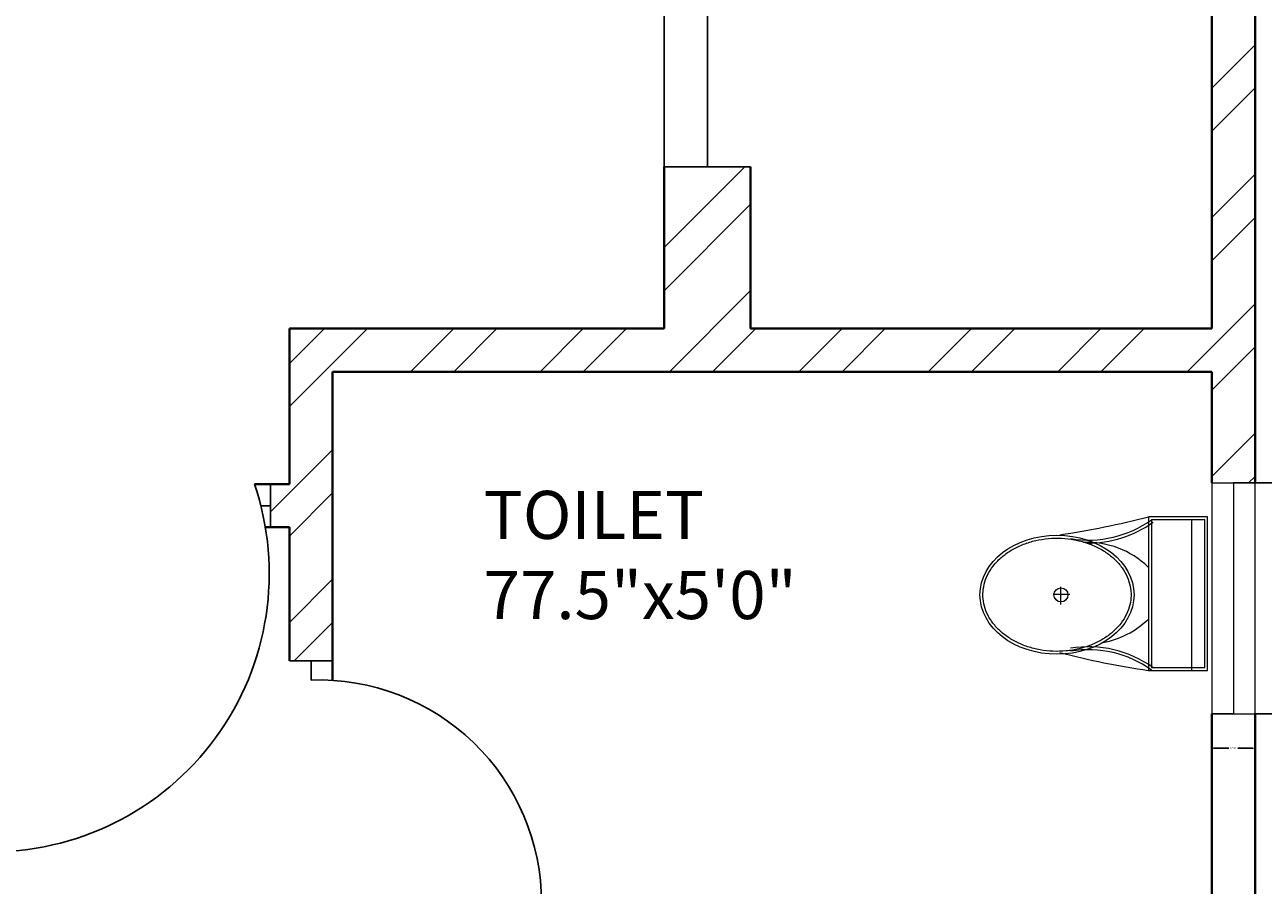
# Model space of a CAD drawing. Units: inches. Extents: x 1601 to 2297, y 1496 to 2631.
# Tile 49 of 57: x 2102 to 2231, y 2237 to 2327. Entities that reach past the tile are written whole.
import ezdxf

# ---------------------------------------------------------------- set-up
doc = ezdxf.new("R2010")
doc.units = ezdxf.units.IN
for name, color, linetype, lineweight in [('A-ANNO-DIMS', 2, 'Continuous', 18), ('A-AREA-IDEN', 7, 'Continuous', 18), ('A-DOOR', 21, 'Continuous', 25), ('A-FLOR-FIXT', 9, 'Continuous', 20), ('A-GLAZ', 161, 'Continuous', 20), ('A-WALL', 7, 'Continuous', 40), ('A-WALL-PATT', 215, 'Continuous', 13)]:
    doc.layers.add(name, color=color, linetype=linetype, lineweight=lineweight)
doc.styles.get("Standard").update_dxf_attribs({"font": 'arial.ttf'})
doc.dimstyles.get("Standard").update_dxf_attribs({"dimtxt": 0.18, "dimasz": 0.18, "dimexe": 0.18, "dimexo": 0.0625, "dimgap": 0.09, "dimtad": 0, "dimtih": 1, "dimtoh": 1, "dimdec": 4, "dimzin": 0, "dimdsep": 46, "dimtxsty": 'Standard', "dimcen": 0.09, "dimadec": 0, "dimazin": 0, "dimtfac": 1, "dimtdec": 4, "dimtofl": 0, "dimtmove": 0, "dimatfit": 3, "dimfxl": 1, "dimtolj": 1, "dimtzin": 0, "dimarcsym": 0})

# ---------------------------------------------------------------- blocks, each defined once
blk = doc.blocks.new('A$C31115884')
for p, q in [((257.5, 466.4), (257.5, 523.2)), ((283.1, 497.7), (223.4, 497.7)), ((0, 200), (0, 0)), ((520, 200), (0, 200)), ((10, 190), (10, 10)), ((510, 190), (10, 190)), ((510, 10), (510, 190)), ((520, 0), (520, 200)), ((510, 54.5), (0, 54.5)), ((10, 10), (510, 10)), ((0, 0), (520, 0))]:
    blk.add_line(p, q)
blk.add_circle((255.6, 496.4), 23.6)
for centre, radius, start, end in [((2777.7, -204.6), 2807, 165.4549, 171.7133), ((-294.5, 403.3), 364.7, 324.2091, 9.3499), ((-294.5, 403.3), 374.7, 324.2091, 9.3499), ((805.8, 403.3), 364.7, 170.6501, 215.7909), ((3237, 905), 2807, 188.2867, 194.5451), ((139.5, 406.2), 293.5, 315.8436, 2.6563), ((805.8, 403.3), 374.7, 179.2036, 215.7909), ((383.6, 406.2), 293.5, 190.2774, 224.1564)]:
    blk.add_arc(centre, radius, start, end)
blk.add_ellipse((256.2, 509.9), major_axis=(0, -260.7), ratio=0.772727)
blk.add_open_spline([(256.2, 259.2), (263.1, 259.2), (270, 259.7), (287.8, 262.3), (298.7, 265.1), (319.9, 273.1), (330.2, 278.4), (350.1, 291.1), (359.7, 298.7), (377.7, 315.9), (386.2, 325.5), (401.7, 346.6), (408.8, 358.1), (421.3, 382.5), (426.8, 395.5), (435.9, 422.4), (439.5, 436.4), (444.8, 465.1), (446.5, 479.7), (447.9, 509.2), (447.6, 524), (445, 553.3), (442.7, 567.8), (436.3, 596), (432.1, 609.7), (421.9, 636), (416, 648.6), (402.5, 672.1), (395, 683), (378.6, 703), (369.8, 712.1), (351.1, 728), (341.3, 734.8), (320.9, 746.2), (310.4, 750.7), (288.9, 757.3), (278, 759.4), (256, 761), (245, 760.6), (223.1, 757.2), (212.3, 754.3), (191.1, 746.1), (180.8, 740.7), (160.9, 727.8), (151.4, 720.1), (133.5, 702.7), (125.1, 693), (109.6, 671.7), (102.6, 660.2), (90.2, 635.7), (84.9, 622.7), (76, 595.6), (72.4, 581.6), (67.2, 552.9), (65.6, 538.2), (64.4, 508.8), (64.8, 494), (67.5, 464.7), (69.9, 450.2), (76.6, 422), (80.8, 408.3), (91.1, 382.2), (97.2, 369.7), (110.8, 346.3), (118.4, 335.4), (134.8, 315.6), (143.7, 306.7), (162.4, 290.9), (172.3, 284.2), (192.8, 273), (203.3, 268.6), (224.8, 262.2), (235.8, 260.2), (249.9, 259.3), (253, 259.2), (256.2, 259.2)], degree=3, knots=[0, 0, 0, 0, 0.110105, 0.110105, 0.285049, 0.285049, 0.459994, 0.459994, 0.634938, 0.634938, 0.809882, 0.809882, 0.984827, 0.984827, 1.159771, 1.159771, 1.334715, 1.334715, 1.50966, 1.50966, 1.684604, 1.684604, 1.859549, 1.859549, 2.034493, 2.034493, 2.209437, 2.209437, 2.384382, 2.384382, 2.559326, 2.559326, 2.73427, 2.73427, 2.909215, 2.909215, 3.084159, 3.084159, 3.259103, 3.259103, 3.434048, 3.434048, 3.608992, 3.608992, 3.783936, 3.783936, 3.958881, 3.958881, 4.133825, 4.133825, 4.30877, 4.30877, 4.483714, 4.483714, 4.658658, 4.658658, 4.833603, 4.833603, 5.008547, 5.008547, 5.183491, 5.183491, 5.358436, 5.358436, 5.53338, 5.53338, 5.708324, 5.708324, 5.883269, 5.883269, 6.058213, 6.058213, 6.233158, 6.233158, 6.283185, 6.283185, 6.283185, 6.283185])
blk = doc.blocks.new('WIN-24IN-JAMB4P5')
for p, q in [((0, 24), (4.5, 24)), ((0, 24), (0, 0)), ((4.5, 24), (2.25, 24)), ((2.25, 24), (2.25, 0)), ((4.5, 24), (4.5, 0)), ((2.25, 0), (0, 0)), ((0, 0), (4.5, 0))]:
    blk.add_line(p, q)
blk = doc.blocks.new('*D22')
at = {"layer": 'A-ANNO-DIMS', "color": 0, "lineweight": -2, "transparency": 16777216}
for p, q in [((2230.6, 2279.25), (2234.32, 2279.25)), ((2234.14, 2279.07), (2234.14, 2267.43)), ((2234.14, 2255.43), (2234.14, 2267.06)), ((2230.6, 2255.25), (2234.32, 2255.25))]:
    blk.add_line(p, q, dxfattribs=at)
at = {"layer": 'A-ANNO-DIMS', "color": 0, "transparency": 16777216}
for points in [[(2234.11, 2279.07), (2234.17, 2279.07), (2234.14, 2279.25)], [(2234.11, 2255.43), (2234.17, 2255.43), (2234.14, 2255.25)]]:
    blk.add_solid(points, dxfattribs=at)
at = {"layer": 'Defpoints', "color": 0, "transparency": 16777216}
for p in [(2230.54, 2279.25), (2234.14, 2279.25), (2230.54, 2255.25)]:
    blk.add_point(p, dxfattribs=at)
at = {"layer": 'A-ANNO-DIMS', "color": 0, "transparency": 16777216, "insert": (2234.14, 2267.25), "char_height": 0.18, "attachment_point": 5}
blk.add_mtext('\\A1;WINDOW 24 TYP.', dxfattribs=at)
blk = doc.blocks.new('*D23')
at = {"layer": 'A-ANNO-DIMS', "color": 0, "lineweight": -2, "transparency": 16777216}
for p, q in [((2226.04, 2255.18), (2226.04, 2251.47)), ((2230.54, 2255.18), (2230.54, 2251.47)), ((2226.22, 2251.65), (2227.83, 2251.65)), ((2230.36, 2251.65), (2228.75, 2251.65))]:
    blk.add_line(p, q, dxfattribs=at)
at = {"layer": 'A-ANNO-DIMS', "color": 0, "transparency": 16777216}
for points in [[(2226.22, 2251.68), (2226.22, 2251.62), (2226.04, 2251.65)], [(2230.36, 2251.68), (2230.36, 2251.62), (2230.54, 2251.65)]]:
    blk.add_solid(points, dxfattribs=at)
at = {"layer": 'Defpoints', "color": 0, "transparency": 16777216}
for p in [(2226.04, 2255.25), (2230.54, 2255.25), (2230.54, 2251.65)]:
    blk.add_point(p, dxfattribs=at)
at = {"layer": 'A-ANNO-DIMS', "color": 0, "transparency": 16777216, "insert": (2228.29, 2251.65), "char_height": 0.18, "attachment_point": 5}
blk.add_mtext('\\A1;5 TYP.', dxfattribs=at)
blk = doc.blocks.new('*D29')
at = {"layer": 'A-ANNO-DIMS', "color": 0, "lineweight": -2, "transparency": 16777216}
for p, q in [((2230.6, 2532.33), (2279.27, 2532.33)), ((2279.09, 2532.15), (2279.09, 2084.01)), ((2279.09, 1635.51), (2279.09, 2083.64)), ((2230.6, 1635.33), (2279.27, 1635.33))]:
    blk.add_line(p, q, dxfattribs=at)
at = {"layer": 'A-ANNO-DIMS', "color": 0, "transparency": 16777216}
for points in [[(2279.06, 2532.15), (2279.12, 2532.15), (2279.09, 2532.33)], [(2279.06, 1635.51), (2279.12, 1635.51), (2279.09, 1635.33)]]:
    blk.add_solid(points, dxfattribs=at)
at = {"layer": 'Defpoints', "color": 0, "transparency": 16777216}
for p in [(2230.54, 2532.33), (2279.09, 2532.33), (2230.54, 1635.33)]:
    blk.add_point(p, dxfattribs=at)
at = {"layer": 'A-ANNO-DIMS', "color": 0, "transparency": 16777216, "insert": (2279.09, 2083.83), "char_height": 0.18, "attachment_point": 5}
blk.add_mtext('\\A1;897', dxfattribs=at)

msp = doc.modelspace()

# ---------------------------------------------------------------- hatches: boundary and pattern name
at = {"layer": 'A-WALL-PATT'}
h = msp.add_hatch(dxfattribs=at)
h.set_pattern_fill('ANSI32', color=256)
h.paths.add_polyline_path([(1842.0336, 2528.0767), (1842.0336, 2532.3254), (1686.0373, 2532.3254), (1686.0373, 2492.9493), (1695.0373, 2492.9493), (1695.0373, 2523.3254), (1827.0373, 2523.3254), (1827.0373, 2416.8254), (1834.6225, 2416.8254), (1834.6225, 2419.0754), (1834.6225, 2421.3254), (1831.5373, 2421.3254), (1831.5373, 2523.3254), (1842.0336, 2523.3254)])
h.paths.add_polyline_path([(1695.0373, 2432.9493), (1686.0373, 2432.9493), (1686.0373, 2325.989), (1695.0373, 2325.989), (1695.0373, 2347.8254), (1827.0373, 2347.8254), (1827.0373, 2287.8254), (1823.2991, 2287.8254), (1823.2991, 2283.3254), (1847.9422, 2283.3254), (1847.9422, 2285.5754), (1847.9422, 2287.8254), (1831.5373, 2287.8254), (1831.5373, 2347.8254), (1846.9946, 2347.8254), (1846.9946, 2350.0754), (1846.9946, 2352.3254), (1695.0373, 2352.3254)])
h.paths.add_polyline_path([(1807.1169, 1573.5395), (2055.0405, 1573.5395), (2055.0405, 1610.6322), (1807.1169, 1610.6322)], flags=9)
h.paths.add_polyline_path([(1841.1631, 1712.7967), (1870.3957, 1712.7967), (1870.3957, 1731.454), (1841.1631, 1731.454)], flags=9)
h.paths.add_polyline_path([(2144.3862, 1772.185), (2191.0233, 1772.185), (2191.0233, 1790.8423), (2144.3862, 1790.8423)], flags=9)
h.paths.add_polyline_path([(2143.0128, 1827.3312), (2177.9958, 1827.3312), (2177.9958, 1845.9886), (2143.0128, 1845.9886)], flags=9)
h.paths.add_polyline_path([(2041.2439, 1833.5691), (2070.8516, 1833.5691), (2070.8516, 1852.2264), (2041.2439, 1852.2264)], flags=9)
h.paths.add_polyline_path([(2097.2791, 1947.0598), (2134.2061, 1947.0598), (2134.2061, 1965.7171), (2097.2791, 1965.7171)], flags=9)
h.paths.add_polyline_path([(2214.995, 1904.3124), (2214.995, 1942.2899), (2196.3376, 1942.2899), (2196.3376, 1904.3124)], flags=9)
h.paths.add_polyline_path([(2186.6284, 2043.8031), (2219.7935, 2043.8031), (2219.7935, 2062.4605), (2186.6284, 2062.4605)], flags=9)
h.paths.add_polyline_path([(2064.0877, 2031.616), (2097.4949, 2031.616), (2097.4949, 2050.2734), (2064.0877, 2050.2734)], flags=9)
h.paths.add_polyline_path([(1973.1349, 1986.0688), (2008.4009, 1986.0688), (2008.4009, 2004.7261), (1973.1349, 2004.7261)], flags=9)
h.paths.add_polyline_path([(1976.3676, 2106.9635), (2005.7469, 2106.9635), (2005.7469, 2125.6209), (1976.3676, 2125.6209)], flags=9)
h.paths.add_polyline_path([(1991.7852, 2180.4863), (2027.0513, 2180.4863), (2027.0513, 2199.1437), (1991.7852, 2199.1437)], flags=9)
h.paths.add_polyline_path([(2106.1801, 2187.9359), (2152.2101, 2187.9359), (2152.2101, 2206.5932), (2106.1801, 2206.5932)], flags=9)
h.paths.add_polyline_path([(2148.6686, 2262.2542), (2182.318, 2262.2542), (2182.318, 2280.9115), (2148.6686, 2280.9115)], flags=9)
h.paths.add_polyline_path([(2041.6327, 2252.8147), (2071.2405, 2252.8147), (2071.2405, 2271.4721), (2041.6327, 2271.4721)], flags=9)
h.paths.add_polyline_path([(2063.9734, 2375.4265), (2100.9004, 2375.4265), (2100.9004, 2394.0839), (2063.9734, 2394.0839)], flags=9)
h.paths.add_polyline_path([(2216.4955, 2330.9748), (2216.4955, 2370.2654), (2197.8381, 2370.2654), (2197.8381, 2330.9748)], flags=9)
h.paths.add_polyline_path([(2179.1416, 2485.8687), (2212.3067, 2485.8687), (2212.3067, 2504.5261), (2179.1416, 2504.5261)], flags=9)
h.paths.add_polyline_path([(2078.7442, 2471.1516), (2112.1514, 2471.1516), (2112.1514, 2489.809), (2078.7442, 2489.809)], flags=9)
h.paths.add_polyline_path([(1915.9631, 2329.4668), (1952.8902, 2329.4668), (1952.8902, 2348.1241), (1915.9631, 2348.1241)], flags=9)
h.paths.add_polyline_path([(1904.3189, 2499.6709), (1940.4512, 2499.6709), (1940.4512, 2518.3282), (1904.3189, 2518.3282)], flags=9)
h.paths.add_polyline_path([(1892.3665, 2100.4595), (1925.6374, 2100.4595), (1925.6374, 2119.1169), (1892.3665, 2119.1169)], flags=9)
h.paths.add_polyline_path([(1909.2984, 1805.9631), (1946.2254, 1805.9631), (1946.2254, 1824.6205), (1909.2984, 1824.6205)], flags=9)
h.paths.add_polyline_path([(1934.6056, 1658.616), (1970.738, 1658.616), (1970.738, 1677.2733), (1934.6056, 1677.2733)], flags=9)
h.paths.add_polyline_path([(1711.2052, 1789.8902), (1750.0456, 1789.8902), (1750.0456, 1808.5476), (1711.2052, 1808.5476)], flags=9)
h.paths.add_polyline_path([(1742.7874, 1854.6743), (1771.9449, 1854.6743), (1771.9449, 1873.3317), (1742.7874, 1873.3317)], flags=9)
h.paths.add_polyline_path([(1807.3592, 1997.7912), (1850.1116, 1997.7912), (1850.1116, 2016.4486), (1807.3592, 2016.4486)], flags=9)
h.paths.add_polyline_path([(1717.4579, 2237.7844), (1760.2103, 2237.7844), (1760.2103, 2256.4417), (1717.4579, 2256.4417)], flags=9)
h.paths.add_polyline_path([(1780.9285, 2324.0623), (1810.086, 2324.0623), (1810.086, 2342.7197), (1780.9285, 2342.7197)], flags=25)
h.paths.add_polyline_path([(1837.696, 2449.2024), (1866.9286, 2449.2024), (1866.9286, 2467.8598), (1837.696, 2467.8598)], flags=9)
h.paths.add_polyline_path([(1712.7752, 2484.9404), (1751.6156, 2484.9404), (1751.6156, 2503.5977), (1712.7752, 2503.5977)], flags=25)
h = msp.add_hatch(dxfattribs=at)
h.set_pattern_fill('ANSI32', color=256)
h.paths.add_polyline_path([(2230.5373, 2532.3254), (2106.0595, 2532.3254), (2106.0595, 2523.3254), (2169.0373, 2523.3254), (2169.0373, 2424.3254), (2091.3989, 2424.3254), (2091.3989, 2419.8254), (2169.0373, 2419.8254), (2169.0373, 2408.1385), (2178.0373, 2408.1385), (2178.0373, 2419.8254), (2181.0581, 2419.8254), (2181.0581, 2422.0754), (2181.0581, 2424.3254), (2178.0373, 2424.3254), (2178.0373, 2523.3254), (2226.0373, 2523.3254), (2226.0373, 2424.3254), (2206.6251, 2424.3254), (2206.6251, 2419.8254), (2226.0373, 2419.8254), (2226.0373, 2299.8254), (2226.0373, 2295.3254), (2178.0373, 2295.3254), (2178.0373, 2312.1385), (2169.0373, 2312.1385), (2169.0373, 2295.3254), (2130.0373, 2295.3254), (2130.0373, 2279.1364), (2128.0593, 2279.1364), (2128.0593, 2274.6364), (2130.0373, 2274.6364), (2130.0373, 2260.7505), (2134.5373, 2260.7505), (2134.5373, 2290.8254), (2226.0373, 2290.8254), (2226.0373, 2279.2475), (2230.5373, 2279.2475), (2230.5373, 2347.8254)])
h.paths.add_polyline_path([(2070.0595, 2532.3254), (2031.0373, 2532.3254), (2031.0373, 2466.3254), (2003.9878, 2466.3254), (2003.9878, 2457.3254), (2031.0373, 2457.3254), (2031.0373, 2419.8254), (2031.0373, 2373.1914), (2035.5373, 2373.1914), (2035.5373, 2419.8254), (2047.3393, 2419.8254), (2047.3393, 2424.3254), (2035.5373, 2424.3254), (2035.5373, 2523.3254), (2070.0595, 2523.3254), (2070.0595, 2527.8254)])
h.paths.add_polyline_path([(1893.0373, 2532.3254), (1866.0336, 2532.3254), (1866.0336, 2523.3254), (1888.5373, 2523.3254), (1888.5373, 2347.8254), (1893.0373, 2347.8254), (1893.0373, 2457.3254), (1907.9878, 2457.3254), (1907.9878, 2466.3254), (1893.0373, 2466.3254)])
h = msp.add_hatch(dxfattribs=at)
h.set_pattern_fill('ANSI32', color=256)
h.paths.add_polyline_path([(1973.9371, 2211.3254), (1893.0373, 2211.3254), (1893.0373, 2287.8254), (1884.6167, 2287.8254), (1884.6167, 2285.5754), (1884.6167, 2283.3254), (1888.5373, 2283.3254), (1888.5373, 2145.3254), (1695.0373, 2145.3254), (1695.0373, 2173.8724), (1690.5373, 2173.8724), (1686.0373, 2173.8724), (1686.0373, 2136.3254), (1722.5687, 2136.3254), (1722.5687, 2117.4352), (1731.5687, 2117.4352), (1731.5687, 2136.3254), (1893.0373, 2136.3254), (1893.0373, 2202.3254), (1959.0373, 2202.3254), (1959.0373, 2182.1303), (1968.0373, 2182.1303), (1968.0373, 2202.3254), (1973.9371, 2202.3254)])
h.paths.add_polyline_path([(2094.0373, 2274.6364), (2096.4294, 2274.6364), (2096.4294, 2276.8864), (2096.4294, 2279.1364), (2094.0373, 2279.1364), (2094.0373, 2290.8254), (2094.0373, 2295.3254), (2089.5373, 2295.3254), (2089.5373, 2230.8254), (2035.5373, 2230.8254), (2035.5373, 2299.8254), (2031.0373, 2299.8254), (2031.0373, 2211.3254), (2023.0065, 2211.3254), (2023.0065, 2202.3254), (2031.0373, 2202.3254), (2031.0373, 2140.8254), (1968.0373, 2140.8254), (1968.0373, 2145.9106), (1963.5373, 2145.9106), (1959.0373, 2145.9106), (1959.0373, 2116.839), (1963.5373, 2116.839), (1968.0373, 2116.839), (1968.0373, 2131.8254), (2031.0373, 2131.8254), (2031.0373, 2094.3254), (2031.0373, 2085.3254), (2031.0373, 2056.8254), (1968.0373, 2056.8254), (1968.0373, 2070.4947), (1963.5373, 2070.4947), (1959.0373, 2070.4947), (1959.0373, 2040.3029), (1968.0373, 2040.3029), (1968.0373, 2047.8254), (2031.0373, 2047.8254), (2031.0373, 1983.3254), (2031.0373, 1978.8254), (2021.1979, 1978.8254), (2021.1979, 1974.3254), (2031.0373, 1974.3254), (2031.0373, 1954.3528), (2035.5373, 1954.3528), (2035.5373, 1974.3254), (2035.5373, 1981.8254), (2055.5513, 1981.8254), (2055.5513, 1986.3254), (2035.5373, 1986.3254), (2035.5373, 2047.8254), (2040.0373, 2047.8254), (2040.0373, 2085.3254), (2040.0373, 2094.3254), (2040.0373, 2140.8254), (2035.5373, 2140.8254), (2035.5373, 2226.3254), (2089.5373, 2226.3254), (2094.0373, 2226.3254)])
h.paths.add_polyline_path([(2226.0373, 2230.8254), (2134.5373, 2230.8254), (2134.5373, 2233.5437), (2130.0373, 2233.5437), (2130.0373, 2226.3254), (2134.5373, 2226.3254), (2226.0373, 2226.3254)])
h.paths.add_polyline_path([(1807.1169, 1573.5395), (2055.0405, 1573.5395), (2055.0405, 1610.6322), (1807.1169, 1610.6322)], flags=9)
h.paths.add_polyline_path([(1841.1631, 1712.7967), (1870.3957, 1712.7967), (1870.3957, 1731.454), (1841.1631, 1731.454)], flags=9)
h.paths.add_polyline_path([(2144.3862, 1772.185), (2191.0233, 1772.185), (2191.0233, 1790.8423), (2144.3862, 1790.8423)], flags=9)
h.paths.add_polyline_path([(2143.0128, 1827.3312), (2177.9958, 1827.3312), (2177.9958, 1845.9886), (2143.0128, 1845.9886)], flags=9)
h.paths.add_polyline_path([(2041.2439, 1833.5691), (2070.8516, 1833.5691), (2070.8516, 1852.2264), (2041.2439, 1852.2264)], flags=9)
h.paths.add_polyline_path([(2097.2791, 1947.0598), (2134.2061, 1947.0598), (2134.2061, 1965.7171), (2097.2791, 1965.7171)], flags=9)
h.paths.add_polyline_path([(2214.995, 1904.3124), (2214.995, 1942.2899), (2196.3376, 1942.2899), (2196.3376, 1904.3124)], flags=9)
h.paths.add_polyline_path([(2186.6284, 2043.8031), (2219.7935, 2043.8031), (2219.7935, 2062.4605), (2186.6284, 2062.4605)], flags=9)
h.paths.add_polyline_path([(2064.0877, 2031.616), (2097.4949, 2031.616), (2097.4949, 2050.2734), (2064.0877, 2050.2734)], flags=9)
h.paths.add_polyline_path([(1973.1349, 1986.0688), (2008.4009, 1986.0688), (2008.4009, 2004.7261), (1973.1349, 2004.7261)], flags=25)
h.paths.add_polyline_path([(1976.3676, 2106.9635), (2005.7469, 2106.9635), (2005.7469, 2125.6209), (1976.3676, 2125.6209)], flags=25)
h.paths.add_polyline_path([(1991.7852, 2180.4863), (2027.0513, 2180.4863), (2027.0513, 2199.1437), (1991.7852, 2199.1437)], flags=25)
h.paths.add_polyline_path([(2106.1801, 2187.9359), (2152.2101, 2187.9359), (2152.2101, 2206.5932), (2106.1801, 2206.5932)], flags=9)
h.paths.add_polyline_path([(2148.6686, 2262.2542), (2182.318, 2262.2542), (2182.318, 2280.9115), (2148.6686, 2280.9115)], flags=9)
h.paths.add_polyline_path([(2041.6327, 2252.8147), (2071.2405, 2252.8147), (2071.2405, 2271.4721), (2041.6327, 2271.4721)], flags=25)
h.paths.add_polyline_path([(2063.9734, 2375.4265), (2100.9004, 2375.4265), (2100.9004, 2394.0839), (2063.9734, 2394.0839)], flags=9)
h.paths.add_polyline_path([(2216.4955, 2330.9748), (2216.4955, 2370.2654), (2197.8381, 2370.2654), (2197.8381, 2330.9748)], flags=9)
h.paths.add_polyline_path([(2179.1416, 2485.8687), (2212.3067, 2485.8687), (2212.3067, 2504.5261), (2179.1416, 2504.5261)], flags=9)
h.paths.add_polyline_path([(2078.7442, 2471.1516), (2112.1514, 2471.1516), (2112.1514, 2489.809), (2078.7442, 2489.809)], flags=9)
h.paths.add_polyline_path([(1915.9631, 2329.4668), (1952.8902, 2329.4668), (1952.8902, 2348.1241), (1915.9631, 2348.1241)], flags=9)
h.paths.add_polyline_path([(1904.3189, 2499.6709), (1940.4512, 2499.6709), (1940.4512, 2518.3282), (1904.3189, 2518.3282)], flags=9)
h.paths.add_polyline_path([(1892.3665, 2100.4595), (1925.6374, 2100.4595), (1925.6374, 2119.1169), (1892.3665, 2119.1169)], flags=9)
h.paths.add_polyline_path([(1909.2984, 1805.9631), (1946.2254, 1805.9631), (1946.2254, 1824.6205), (1909.2984, 1824.6205)], flags=9)
h.paths.add_polyline_path([(1934.6056, 1658.616), (1970.738, 1658.616), (1970.738, 1677.2733), (1934.6056, 1677.2733)], flags=9)
h.paths.add_polyline_path([(1711.2052, 1789.8902), (1750.0456, 1789.8902), (1750.0456, 1808.5476), (1711.2052, 1808.5476)], flags=9)
h.paths.add_polyline_path([(1742.7874, 1854.6743), (1771.9449, 1854.6743), (1771.9449, 1873.3317), (1742.7874, 1873.3317)], flags=9)
h.paths.add_polyline_path([(1807.3592, 1997.7912), (1850.1116, 1997.7912), (1850.1116, 2016.4486), (1807.3592, 2016.4486)], flags=9)
h.paths.add_polyline_path([(1717.4579, 2237.7844), (1760.2103, 2237.7844), (1760.2103, 2256.4417), (1717.4579, 2256.4417)], flags=25)
h.paths.add_polyline_path([(1780.9285, 2324.0623), (1810.086, 2324.0623), (1810.086, 2342.7197), (1780.9285, 2342.7197)], flags=9)
h.paths.add_polyline_path([(1837.696, 2449.2024), (1866.9286, 2449.2024), (1866.9286, 2467.8598), (1837.696, 2467.8598)], flags=9)
h.paths.add_polyline_path([(1712.7752, 2484.9404), (1751.6156, 2484.9404), (1751.6156, 2503.5977), (1712.7752, 2503.5977)], flags=9)
h = msp.add_hatch(dxfattribs=at)
h.set_pattern_fill('ANSI32', color=256)
h.paths.add_polyline_path([(2230.5373, 1861.8254), (2182.5373, 1861.8254), (2182.5373, 1885.3637), (2178.0373, 1885.3637), (2178.0373, 1861.8254), (2166.0373, 1861.8254), (2134.5373, 1861.8254), (2130.0373, 1861.8254), (2130.0373, 1841.4682), (2126.8833, 1841.4682), (2126.8833, 1836.9682), (2130.0373, 1836.9682), (2130.0373, 1822.7302), (2134.5373, 1822.7302), (2134.5373, 1857.3254), (2166.0373, 1857.3254), (2226.0373, 1857.3254), (2226.0373, 1846.1155), (2230.5373, 1846.1155)])
h.paths.add_polyline_path([(2226.0373, 1797.3254), (2134.5373, 1797.3254), (2134.5373, 1800.6636), (2132.2873, 1800.6636), (2130.0373, 1800.6636), (2130.0373, 1797.3254), (2130.0373, 1792.8254), (2167.7264, 1792.8254), (2226.0373, 1792.8254)])
h.paths.add_polyline_path([(2230.5373, 1822.1155), (2226.0373, 1822.1155), (2226.0373, 1760.8563), (2230.5373, 1760.8563)])
h.paths.add_polyline_path([(2230.5373, 1700.8563), (2226.0373, 1700.8563), (2226.0373, 1644.3254), (2140.2517, 1644.3254), (2140.2517, 1635.3254), (2230.5373, 1635.3254)])
h.paths.add_polyline_path([(2080.2517, 1639.8254), (2080.2517, 1644.3254), (2035.5373, 1644.3254), (2035.5373, 1792.8254), (2094.0373, 1792.8254), (2094.0373, 1797.3254), (2094.0373, 1836.9682), (2097.1057, 1836.9682), (2097.1057, 1839.2182), (2097.1057, 1841.4682), (2094.0373, 1841.4682), (2094.0373, 1862.2276), (2089.5373, 1862.2276), (2089.5373, 1797.3254), (2035.5373, 1797.3254), (2035.5373, 1857.3254), (2035.5373, 1885.0916), (2031.0373, 1885.0916), (2031.0373, 1710.3254), (2012.329, 1710.3254), (2012.329, 1701.3254), (2031.0373, 1701.3254), (2031.0373, 1644.3254), (2031.0373, 1635.3254), (2080.2517, 1635.3254)])
h.paths.add_polyline_path([(1836.0373, 1653.2033), (1842.6171, 1653.2033), (1842.6171, 1657.7033), (1842.6171, 1662.2033), (1831.5373, 1662.2033), (1831.5373, 1764.2033), (1835.3881, 1764.2033), (1835.3881, 1766.4533), (1835.3881, 1768.7033), (1831.5373, 1768.7033), (1827.0373, 1768.7033), (1827.0373, 1662.2033), (1827.0373, 1635.3254), (1836.0373, 1635.3254)])
h.paths.add_polyline_path([(1893.0373, 1701.3254), (1907.193, 1701.3254), (1907.193, 1705.8254), (1907.193, 1710.3254), (1893.0373, 1710.3254), (1893.0373, 1819.8254), (1882.6444, 1819.8254), (1882.6444, 1817.5754), (1882.6444, 1815.3254), (1888.5373, 1815.3254), (1888.5373, 1662.2033), (1884.0373, 1662.2033), (1866.6171, 1662.2033), (1866.6171, 1653.2033), (1882.391, 1653.2033), (1884.0373, 1653.2033), (1884.0373, 1635.3254), (1893.0373, 1635.3254)])
h.paths.add_polyline_path([(1739.3335, 1639.8254), (1739.3335, 1644.3254), (1695.0373, 1644.3254), (1695.0373, 1702.0135), (1690.5373, 1702.0135), (1686.0373, 1702.0135), (1686.0373, 1635.3254), (1739.3335, 1635.3254)])
h.paths.add_polyline_path([(1827.0373, 1644.3254), (1799.3335, 1644.3254), (1799.3335, 1635.3254), (1827.0373, 1635.3254)])
h.paths.add_polyline_path([(1695.0373, 1815.3254), (1849.2759, 1815.3254), (1849.2759, 1819.8254), (1807.5373, 1819.8254), (1807.5373, 1879.8254), (1851.1533, 1879.8254), (1851.1533, 1882.0754), (1851.1533, 1884.3254), (1799.3405, 1884.3254), (1799.3405, 1882.0754), (1799.3405, 1879.8254), (1803.0373, 1879.8254), (1803.0373, 1819.8254), (1695.0373, 1819.8254), (1695.0373, 1835.0458), (1690.5373, 1835.0458), (1686.0373, 1835.0458), (1686.0373, 1766.1753), (1695.0373, 1766.1753)])
h.paths.add_polyline_path([(1775.8157, 1884.3254), (1695.0373, 1884.3254), (1695.0373, 1912.9526), (1690.5373, 1912.9526), (1686.0373, 1912.9526), (1686.0373, 1859.0458), (1695.0373, 1859.0458), (1695.0373, 1879.8254), (1775.8157, 1879.8254)])
h.paths.add_polyline_path([(1893.0373, 2031.3254), (1731.5687, 2031.3254), (1731.5687, 2057.4352), (1722.5687, 2057.4352), (1722.5687, 2031.3254), (1686.0373, 2031.3254), (1686.0373, 1972.9526), (1695.0373, 1972.9526), (1695.0373, 2022.3254), (1888.5373, 2022.3254), (1888.5373, 1884.3254), (1883.4996, 1884.3254), (1883.4996, 1879.8254), (1893.0373, 1879.8254), (1893.0373, 1974.3254), (1976.6199, 1974.3254), (1976.6199, 1978.8254), (1968.0373, 1978.8254), (1968.0373, 1983.3254), (1968.0373, 2008.4756), (1963.5373, 2008.4756), (1959.0373, 2008.4756), (1959.0373, 1983.3254), (1893.0373, 1983.3254)])
h.paths.add_polyline_path([(2230.5373, 2140.4745), (2226.0373, 2140.4745), (2226.0373, 2094.3254), (2040.0373, 2094.3254), (2040.0373, 2085.3254), (2178.0373, 2085.3254), (2178.0373, 2065.6965), (2182.5373, 2065.6965), (2182.5373, 2085.3254), (2226.0373, 2085.3254), (2226.0373, 1986.3254), (2211.2679, 1986.3254), (2211.2679, 1981.8254), (2230.5373, 1981.8254)])
h.paths.add_polyline_path([(2187.6292, 1986.3254), (2182.5373, 1986.3254), (2182.5373, 2029.6965), (2178.0373, 2029.6965), (2178.0373, 1986.3254), (2099.05, 1986.3254), (2099.05, 1981.8254), (2178.0373, 1981.8254), (2178.0373, 1969.3637), (2182.5373, 1969.3637), (2182.5373, 1981.8254), (2187.6292, 1981.8254), (2187.6292, 1984.0754)])
h.paths.add_polyline_path([(1807.1169, 1573.5395), (2055.0405, 1573.5395), (2055.0405, 1610.6322), (1807.1169, 1610.6322)], flags=9)
h.paths.add_polyline_path([(1841.1631, 1712.7967), (1870.3957, 1712.7967), (1870.3957, 1731.454), (1841.1631, 1731.454)], flags=9)
h.paths.add_polyline_path([(2144.3862, 1772.185), (2191.0233, 1772.185), (2191.0233, 1790.8423), (2144.3862, 1790.8423)], flags=9)
h.paths.add_polyline_path([(2143.0128, 1827.3312), (2177.9958, 1827.3312), (2177.9958, 1845.9886), (2143.0128, 1845.9886)], flags=25)
h.paths.add_polyline_path([(2041.2439, 1833.5691), (2070.8516, 1833.5691), (2070.8516, 1852.2264), (2041.2439, 1852.2264)], flags=25)
h.paths.add_polyline_path([(2097.2791, 1947.0598), (2134.2061, 1947.0598), (2134.2061, 1965.7171), (2097.2791, 1965.7171)], flags=9)
h.paths.add_polyline_path([(2214.995, 1904.3124), (2214.995, 1942.2899), (2196.3376, 1942.2899), (2196.3376, 1904.3124)], flags=9)
h.paths.add_polyline_path([(2186.6284, 2043.8031), (2219.7935, 2043.8031), (2219.7935, 2062.4605), (2186.6284, 2062.4605)], flags=25)
h.paths.add_polyline_path([(2064.0877, 2031.616), (2097.4949, 2031.616), (2097.4949, 2050.2734), (2064.0877, 2050.2734)], flags=25)
h.paths.add_polyline_path([(1973.1349, 1986.0688), (2008.4009, 1986.0688), (2008.4009, 2004.7261), (1973.1349, 2004.7261)], flags=9)
h.paths.add_polyline_path([(1976.3676, 2106.9635), (2005.7469, 2106.9635), (2005.7469, 2125.6209), (1976.3676, 2125.6209)], flags=9)
h.paths.add_polyline_path([(1991.7852, 2180.4863), (2027.0513, 2180.4863), (2027.0513, 2199.1437), (1991.7852, 2199.1437)], flags=9)
h.paths.add_polyline_path([(2106.1801, 2187.9359), (2152.2101, 2187.9359), (2152.2101, 2206.5932), (2106.1801, 2206.5932)], flags=9)
h.paths.add_polyline_path([(2148.6686, 2262.2542), (2182.318, 2262.2542), (2182.318, 2280.9115), (2148.6686, 2280.9115)], flags=9)
h.paths.add_polyline_path([(2041.6327, 2252.8147), (2071.2405, 2252.8147), (2071.2405, 2271.4721), (2041.6327, 2271.4721)], flags=9)
h.paths.add_polyline_path([(2063.9734, 2375.4265), (2100.9004, 2375.4265), (2100.9004, 2394.0839), (2063.9734, 2394.0839)], flags=9)
h.paths.add_polyline_path([(2216.4955, 2330.9748), (2216.4955, 2370.2654), (2197.8381, 2370.2654), (2197.8381, 2330.9748)], flags=9)
h.paths.add_polyline_path([(2179.1416, 2485.8687), (2212.3067, 2485.8687), (2212.3067, 2504.5261), (2179.1416, 2504.5261)], flags=9)
h.paths.add_polyline_path([(2078.7442, 2471.1516), (2112.1514, 2471.1516), (2112.1514, 2489.809), (2078.7442, 2489.809)], flags=9)
h.paths.add_polyline_path([(1915.9631, 2329.4668), (1952.8902, 2329.4668), (1952.8902, 2348.1241), (1915.9631, 2348.1241)], flags=9)
h.paths.add_polyline_path([(1904.3189, 2499.6709), (1940.4512, 2499.6709), (1940.4512, 2518.3282), (1904.3189, 2518.3282)], flags=9)
h.paths.add_polyline_path([(1892.3665, 2100.4595), (1925.6374, 2100.4595), (1925.6374, 2119.1169), (1892.3665, 2119.1169)], flags=9)
h.paths.add_polyline_path([(1909.2984, 1805.9631), (1946.2254, 1805.9631), (1946.2254, 1824.6205), (1909.2984, 1824.6205)], flags=9)
h.paths.add_polyline_path([(1934.6056, 1658.616), (1970.738, 1658.616), (1970.738, 1677.2733), (1934.6056, 1677.2733)], flags=9)
h.paths.add_polyline_path([(1711.2052, 1789.8902), (1750.0456, 1789.8902), (1750.0456, 1808.5476), (1711.2052, 1808.5476)], flags=25)
h.paths.add_polyline_path([(1742.7874, 1854.6743), (1771.9449, 1854.6743), (1771.9449, 1873.3317), (1742.7874, 1873.3317)], flags=25)
h.paths.add_polyline_path([(1807.3592, 1997.7912), (1850.1116, 1997.7912), (1850.1116, 2016.4486), (1807.3592, 2016.4486)], flags=25)
h.paths.add_polyline_path([(1717.4579, 2237.7844), (1760.2103, 2237.7844), (1760.2103, 2256.4417), (1717.4579, 2256.4417)], flags=9)
h.paths.add_polyline_path([(1780.9285, 2324.0623), (1810.086, 2324.0623), (1810.086, 2342.7197), (1780.9285, 2342.7197)], flags=9)
h.paths.add_polyline_path([(1837.696, 2449.2024), (1866.9286, 2449.2024), (1866.9286, 2467.8598), (1837.696, 2467.8598)], flags=9)
h.paths.add_polyline_path([(1712.7752, 2484.9404), (1751.6156, 2484.9404), (1751.6156, 2503.5977), (1712.7752, 2503.5977)], flags=9)

# ---------------------------------------------------------------- linework, layer by layer
at = {"layer": 'A-DOOR'}
for p, q in [((2169.0373, 2375.3908), (2169.0373, 2312.1385)), ((2173.5373, 2348.1385), (2173.5373, 2312.1385)), ((2173.5373, 2312.1385), (2169.0373, 2312.1385)), ((2169.0373, 2312.1385), (2178.0373, 2312.1385)), ((2178.0373, 2312.1385), (2178.0373, 2312.1385)), ((2128.0593, 2279.1364), (2128.0593, 2274.6364)), ((2128.0593, 2276.8864), (2127.0593, 2276.8864)), ((2128.0593, 2274.6364), (2128.0593, 2276.8864)), ((2130.0373, 2260.7505), (2134.5373, 2260.7505)), ((2134.5373, 2260.7505), (2132.2873, 2260.7505)), ((2132.2873, 2260.7505), (2132.2873, 2258.7505))]:
    msp.add_line(p, q, dxfattribs=at)
for centre, radius, start, end in [((2098.9928, 2269.8227), 28.9418, 268.884453, 18.772337), ((2133.0674, 2235.5437), 23.2199, 360, 91.925269)]:
    msp.add_arc(centre, radius, start, end, dxfattribs=at)
at = {"layer": 'A-WALL'}
for p, q in [((2226.0373, 2419.8254), (2226.0373, 2299.8254)), ((2226.0373, 2352.3254), (2226.0373, 2299.8254)), ((2230.5373, 2347.8254), (2230.5373, 2279.2475)), ((2169.0373, 2312.1385), (2169.0373, 2295.3254)), ((2178.0373, 2295.3254), (2178.0373, 2312.1385)), ((2226.0373, 2299.8254), (2226.0373, 2295.3254)), ((2169.0373, 2295.3254), (2130.0373, 2295.3254)), ((2130.0373, 2279.1364), (2130.0373, 2295.3254)), ((2226.0373, 2295.3254), (2178.0373, 2295.3254)), ((2134.5373, 2290.8254), (2226.0373, 2290.8254)), ((2134.5373, 2290.8254), (2134.5373, 2258.717)), ((2226.0373, 2290.8254), (2226.0373, 2279.2475)), ((2126.395, 2279.1364), (2130.0373, 2279.1364)), ((2130.0373, 2274.6364), (2127.5315, 2274.6364)), ((2130.0373, 2260.7505), (2130.0373, 2274.6364)), ((2226.0373, 2255.2475), (2226.0373, 2200.4745)), ((2230.5373, 2255.2475), (2230.5373, 2200.4745))]:
    msp.add_line(p, q, dxfattribs=at)

# ---------------------------------------------------------------- block references
at = {"layer": 'A-FLOR-FIXT', "xscale": 0.0307498789965588, "yscale": 0.0307498789965588, "zscale": 0.0307498789965588, "rotation": 89.99999999999999}
msp.add_blockref('A$C31115884', (2225.6064, 2259.7429), dxfattribs=at)
at = {"layer": 'A-GLAZ'}
msp.add_blockref('WIN-24IN-JAMB4P5', (2226.037, 2255.247), dxfattribs=at)

# ---------------------------------------------------------------- texts
at = {"layer": 'A-AREA-IDEN', "insert": (2150.2494, 2278.4269), "char_height": 5, "attachment_point": 1}
msp.add_mtext_dynamic_manual_height_columns('TOILET\\P77.5"x5\'0"', width=55.591251, gutter_width=12.5, heights=[0], dxfattribs=at)

# ---------------------------------------------------------------- dimensions: what is measured, and where the dimension line sits
at = {"layer": 'A-ANNO-DIMS'}
dim = msp.add_linear_dim(base=(2279.0873, 2532.3254), p1=(2230.5373, 1635.3254), p2=(2230.5373, 2532.3254), angle=90, dimstyle='Standard', override={"dimdec": 0, "dimlfac": 1, "dimrnd": 0, "dimzin": 0, "dimdsep": 46, "dimlunit": 2}, dxfattribs=at)
dim.commit()
dim.dimension.update_dxf_attribs({"geometry": '*D29', "text_midpoint": (2279.0873, 2083.8254)})
dim = msp.add_linear_dim(base=(2234.1373, 2279.2475), p1=(2230.5373, 2255.2475), p2=(2230.5373, 2279.2475), angle=90, text='WINDOW <> TYP.', dimstyle='Standard', override={"dimdec": 0, "dimlfac": 1, "dimrnd": 0, "dimzin": 0, "dimdsep": 46, "dimlunit": 2}, dxfattribs=at)
dim.commit()
dim.dimension.update_dxf_attribs({"geometry": '*D22', "text_midpoint": (2234.1373, 2267.2475)})
dim = msp.add_linear_dim(base=(2230.5373150195, 2251.6474520939), p1=(2226.0373150195, 2255.2474520939), p2=(2230.5373150195, 2255.2474520939), text='<> TYP.', dimstyle='Standard', override={"dimdec": 0, "dimlfac": 1, "dimrnd": 0, "dimzin": 0, "dimdsep": 46, "dimlunit": 2}, dxfattribs=at)
dim.commit()
dim.dimension.update_dxf_attribs({"geometry": '*D23', "text_midpoint": (2228.2873150195, 2251.6474520939)})

doc.saveas('drawing.dxf')
